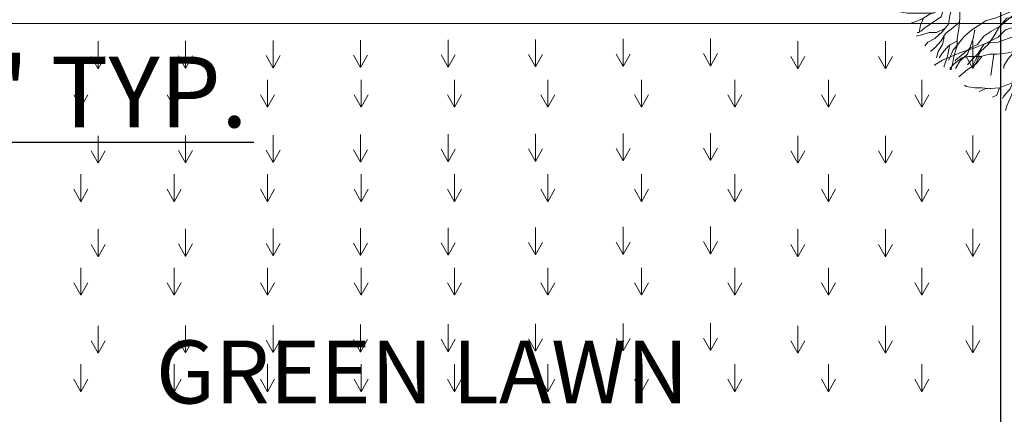
# Model space of a CAD drawing. Units: millimetres. Extents: x 595116 to 630915, y 909473 to 920225.
# Tile 66 of 134: x 629619 to 629744, y 919216 to 919267. Entities that reach past the tile are written whole.
import ezdxf

# ---------------------------------------------------------------- set-up
doc = ezdxf.new("R2010")
doc.units = ezdxf.units.MM
for name, color, linetype, lineweight in [('A-AREA-IDEN', 7, 'Continuous', 20), ('Dimension', 3, 'Continuous', 18), ('L-PLNT', 85, 'Continuous', 13)]:
    doc.layers.add(name, color=color, linetype=linetype, lineweight=lineweight)
doc.styles.get("Standard").update_dxf_attribs({"font": 'arial.ttf'})
doc.dimstyles.new('ISO-25', dxfattribs={"dimtxt": 9, "dimasz": 6, "dimexe": 1.25, "dimexo": 0.625, "dimtad": 1, "dimlunit": 4, "dimtxsty": 'Standard', "dimcen": 2.5, "dimadec": 0, "dimazin": 0, "dimtfac": 1, "dimtmove": 0, "dimatfit": 3, "dimfxl": 1, "dimarcsym": 0})

# ---------------------------------------------------------------- blocks, each defined once
blk = doc.blocks.new('A$C143125F4')
for p, q in [((2.883, 4.834), (2.883, 5.044)), ((2.155, 4.937), (2.117, 4.982)), ((2.21, 4.834), (2.155, 4.937)), ((2.407, 4.879), (2.429, 4.937)), ((2.516, 4.834), (2.538, 4.91)), ((2.538, 4.82), (2.571, 5)), ((2.571, 5), (2.555, 4.982)), ((2.757, 4.892), (2.735, 4.955)), ((1.712, 4.431), (1.712, 4.82)), ((1.822, 4.368), (1.822, 4.802)), ((1.898, 4.776), (1.898, 4.865)), ((1.937, 4.713), (1.991, 4.82)), ((1.991, 4.82), (2.008, 4.865)), ((2.21, 4.744), (2.062, 4.865)), ((2.281, 4.744), (2.21, 4.834)), ((2.298, 4.847), (2.281, 4.892)), ((2.352, 4.758), (2.298, 4.847)), ((2.391, 4.789), (2.407, 4.879)), ((2.391, 4.681), (2.391, 4.789)), ((2.516, 4.52), (2.516, 4.834)), ((2.538, 4.547), (2.538, 4.82)), ((2.648, 4.865), (2.626, 4.892)), ((2.681, 4.776), (2.648, 4.865)), ((2.79, 4.776), (2.757, 4.892)), ((2.867, 4.699), (2.883, 4.834)), ((2.899, 4.699), (2.921, 4.789)), ((2.921, 4.789), (2.96, 4.879)), ((2.96, 4.879), (2.96, 4.892)), ((3.014, 4.713), (3.031, 4.802)), ((3.031, 4.802), (3.031, 4.865)), ((3.047, 4.668), (3.069, 4.789)), ((3.069, 4.789), (3.085, 4.847)), ((3.124, 4.731), (3.124, 4.802)), ((3.178, 4.744), (3.178, 4.82)), ((1.461, 4.681), (1.461, 4.699)), ((1.493, 4.592), (1.461, 4.681)), ((1.625, 4.655), (1.586, 4.699)), ((1.915, 4.668), (1.898, 4.776)), ((1.898, 4.623), (1.937, 4.713)), ((2.298, 4.668), (2.21, 4.744)), ((2.352, 4.578), (2.298, 4.668)), ((2.391, 4.668), (2.352, 4.758)), ((2.429, 4.565), (2.391, 4.668)), ((2.719, 4.681), (2.681, 4.776)), ((2.757, 4.592), (2.719, 4.681)), ((2.812, 4.637), (2.79, 4.776)), ((2.867, 4.431), (2.867, 4.699)), ((2.883, 4.547), (2.899, 4.699)), ((2.976, 4.61), (3.014, 4.713)), ((3.031, 4.578), (3.047, 4.668)), ((3.102, 4.637), (3.124, 4.731)), ((3.156, 4.655), (3.178, 4.744)), ((3.288, 4.637), (3.304, 4.731)), ((3.342, 4.655), (3.375, 4.699)), ((3.414, 4.592), (3.468, 4.681)), ((3.485, 4.623), (3.485, 4.681)), ((1.275, 4.534), (1.258, 4.61)), ((1.368, 4.61), (1.368, 4.623)), ((1.422, 4.52), (1.368, 4.61)), ((1.532, 4.502), (1.493, 4.592)), ((1.658, 4.565), (1.625, 4.655)), ((1.712, 4.475), (1.658, 4.565)), ((1.882, 4.534), (1.898, 4.623)), ((2.429, 4.489), (2.352, 4.578)), ((2.462, 4.444), (2.429, 4.565)), ((2.5, 4.099), (2.538, 4.547)), ((2.79, 4.413), (2.757, 4.592)), ((2.828, 4.296), (2.812, 4.637)), ((2.867, 4.457), (2.883, 4.547)), ((2.976, 4.52), (2.976, 4.61)), ((3.069, 4.457), (3.102, 4.547)), ((3.102, 4.547), (3.102, 4.637)), ((3.14, 4.565), (3.156, 4.655)), ((3.14, 4.413), (3.14, 4.565)), ((3.249, 4.457), (3.266, 4.547)), ((3.266, 4.547), (3.288, 4.637)), ((3.288, 4.565), (3.342, 4.655)), ((3.375, 4.502), (3.414, 4.592)), ((3.507, 4.534), (3.485, 4.623)), ((3.539, 4.444), (3.561, 4.547)), ((3.561, 4.547), (3.578, 4.637)), ((3.578, 4.637), (3.578, 4.655)), ((3.632, 4.534), (3.632, 4.623)), ((1.111, 4.399), (1.039, 4.444)), ((1.056, 4.399), (1.039, 4.431)), ((1.078, 4.457), (1.165, 4.444)), ((1.165, 4.444), (1.258, 4.413)), ((1.368, 4.489), (1.275, 4.534)), ((1.406, 4.341), (1.368, 4.489)), ((1.461, 4.431), (1.422, 4.52)), ((1.548, 4.368), (1.461, 4.431)), ((1.548, 4.413), (1.532, 4.502)), ((1.734, 4.386), (1.712, 4.475)), ((1.822, 4.444), (1.882, 4.534)), ((2.445, 4.399), (2.429, 4.489)), ((2.484, 4.354), (2.462, 4.444)), ((2.5, 4.431), (2.516, 4.52)), ((2.5, 3.458), (2.5, 4.431)), ((2.845, 4.162), (2.867, 4.431)), ((3.047, 4.368), (3.069, 4.457)), ((3.249, 4.368), (3.249, 4.457)), ((3.321, 4.413), (3.375, 4.502)), ((3.507, 4.399), (3.507, 4.534)), ((3.523, 4.31), (3.539, 4.444)), ((3.649, 4.444), (3.632, 4.534)), ((3.649, 4.189), (3.649, 4.444)), ((3.704, 4.413), (3.725, 4.502)), ((3.725, 4.502), (3.725, 4.534)), ((3.797, 4.278), (3.797, 4.489)), ((3.835, 4.386), (3.851, 4.475)), ((3.851, 4.475), (3.868, 4.489)), ((0.946, 4.341), (0.914, 4.386)), ((0.985, 4.251), (0.946, 4.341)), ((1.078, 4.265), (0.985, 4.341)), ((1.094, 4.31), (1.056, 4.399)), ((1.149, 4.22), (1.094, 4.31)), ((1.297, 4.31), (1.111, 4.399)), ((1.258, 4.413), (1.351, 4.386)), ((1.384, 4.278), (1.297, 4.31)), ((1.351, 4.386), (1.439, 4.31)), ((1.439, 4.31), (1.515, 4.22)), ((1.57, 4.296), (1.548, 4.413)), ((1.625, 4.207), (1.57, 4.296)), ((1.767, 4.296), (1.734, 4.386)), ((1.805, 4.207), (1.767, 4.296)), ((1.805, 4.251), (1.822, 4.368)), ((2.5, 4.278), (2.445, 4.399)), ((2.5, 4.265), (2.484, 4.354)), ((2.812, 4.31), (2.79, 4.413)), ((2.828, 4.22), (2.812, 4.31)), ((2.845, 4.207), (2.828, 4.296)), ((3.014, 4.278), (3.047, 4.368)), ((3.069, 4.233), (3.102, 4.323)), ((3.102, 4.323), (3.14, 4.413)), ((3.14, 4.233), (3.211, 4.341)), ((3.211, 4.341), (3.321, 4.413)), ((3.523, 4.31), (3.507, 4.399)), ((3.539, 4.189), (3.523, 4.31)), ((3.671, 4.233), (3.704, 4.413)), ((3.797, 4.278), (3.835, 4.386)), ((3.906, 4.278), (3.961, 4.341)), ((3.961, 4.233), (3.999, 4.323)), ((3.999, 4.323), (3.999, 4.341)), ((0.837, 4.144), (0.766, 4.189)), ((0.837, 4.22), (0.804, 4.265)), ((0.93, 4.175), (0.837, 4.22)), ((1.039, 4.13), (0.93, 4.175)), ((1.039, 4.144), (0.985, 4.251)), ((1.165, 4.175), (1.078, 4.265)), ((1.22, 4.086), (1.165, 4.175)), ((1.493, 4.233), (1.384, 4.278)), ((1.548, 4.144), (1.493, 4.233)), ((1.515, 4.22), (1.603, 4.175)), ((1.603, 4.175), (1.658, 4.086)), ((1.658, 4.099), (1.625, 4.207)), ((1.805, 3.906), (1.805, 4.251)), ((2.516, 4.009), (2.5, 4.278)), ((2.845, 4.117), (2.828, 4.22)), ((2.96, 4.086), (2.992, 4.175)), ((2.992, 4.175), (3.014, 4.278)), ((3.047, 4.189), (3.14, 4.233)), ((3.047, 4.144), (3.069, 4.233)), ((3.561, 4.099), (3.539, 4.189)), ((3.632, 4.144), (3.671, 4.233)), ((3.725, 4.117), (3.813, 4.207)), ((3.78, 4.162), (3.797, 4.278)), ((3.813, 4.207), (3.906, 4.278)), ((3.944, 4.175), (4.037, 4.251)), ((3.944, 4.144), (3.961, 4.233)), ((3.961, 3.92), (4.125, 4.189)), ((4.037, 4.251), (4.037, 4.278)), ((4.125, 4.251), (4.054, 4.162)), ((0.563, 4.027), (0.525, 4.072)), ((0.689, 4.117), (0.673, 4.13)), ((0.782, 4.072), (0.689, 4.117)), ((0.766, 4.086), (0.711, 4.144)), ((0.821, 3.996), (0.766, 4.086)), ((0.968, 4.072), (0.782, 4.072)), ((0.93, 4.099), (0.837, 4.144)), ((1.149, 4.054), (0.968, 4.072)), ((1.132, 4.086), (1.039, 4.13)), ((1.22, 4.054), (1.132, 4.086)), ((1.313, 4.054), (1.22, 4.086)), ((1.313, 4.041), (1.22, 4.054)), ((1.641, 4.054), (1.548, 4.144)), ((1.679, 3.938), (1.641, 4.054)), ((1.658, 4.086), (1.734, 3.996)), ((2.5, 3.996), (2.5, 4.099)), ((2.828, 3.83), (2.845, 4.162)), ((2.938, 3.983), (2.96, 4.086)), ((3.031, 4.054), (3.047, 4.144)), ((3.031, 3.965), (3.031, 4.054)), ((3.594, 4.009), (3.561, 4.099)), ((3.594, 3.875), (3.632, 4.144)), ((3.632, 4.099), (3.725, 4.117)), ((3.922, 4.041), (3.944, 4.144)), ((3.999, 4.072), (3.922, 3.983)), ((4.054, 4.162), (3.999, 4.072)), ((4.147, 3.965), (4.218, 4.054)), ((4.218, 4.054), (4.234, 4.086)), ((0.509, 3.92), (0.509, 3.938)), ((0.602, 3.951), (0.547, 3.996)), ((0.656, 3.983), (0.563, 4.027)), ((0.618, 3.92), (0.563, 3.983)), ((0.635, 3.862), (0.602, 3.951)), ((0.821, 3.965), (0.656, 3.983)), ((0.892, 3.906), (0.821, 3.996)), ((1.406, 4.009), (1.313, 4.041)), ((1.493, 3.996), (1.406, 4.009)), ((1.586, 3.965), (1.493, 3.996)), ((1.679, 3.951), (1.586, 3.965)), ((1.696, 3.817), (1.679, 3.938)), ((1.734, 3.996), (1.789, 3.906)), ((2.883, 3.893), (2.938, 3.983)), ((3.047, 3.875), (3.031, 3.965)), ((3.616, 3.92), (3.594, 4.009)), ((3.922, 3.983), (3.835, 3.92)), ((3.89, 3.951), (3.922, 4.041)), ((4.108, 3.875), (4.147, 3.965)), ((4.147, 3.92), (4.218, 4.009)), ((4.218, 4.009), (4.234, 4.027)), ((4.311, 3.92), (4.344, 3.951)), ((0.47, 3.817), (0.438, 3.83)), ((0.563, 3.741), (0.47, 3.817)), ((0.563, 3.83), (0.509, 3.92)), ((0.602, 3.727), (0.563, 3.83)), ((0.728, 3.862), (0.618, 3.92)), ((0.689, 3.772), (0.635, 3.862)), ((0.914, 3.772), (0.728, 3.862)), ((0.93, 3.817), (0.892, 3.906)), ((0.985, 3.727), (0.93, 3.817)), ((1.734, 3.665), (1.696, 3.817)), ((1.789, 3.906), (1.805, 3.785)), ((2.812, 3.785), (2.883, 3.893)), ((3.14, 3.862), (3.047, 3.875)), ((3.233, 3.83), (3.14, 3.862)), ((3.321, 3.799), (3.233, 3.83)), ((3.578, 3.785), (3.594, 3.875)), ((3.78, 3.83), (3.687, 3.799)), ((3.758, 3.754), (3.961, 3.92)), ((3.835, 3.92), (3.78, 3.83)), ((3.961, 3.785), (4.07, 3.83)), ((4.07, 3.83), (4.147, 3.92)), ((4.125, 3.785), (4.234, 3.83)), ((4.234, 3.83), (4.311, 3.92)), ((4.344, 3.785), (4.437, 3.862)), ((4.437, 3.862), (4.437, 3.893)), ((0.252, 3.696), (0.252, 3.727)), ((0.345, 3.682), (0.252, 3.696)), ((0.492, 3.665), (0.345, 3.682)), ((0.656, 3.696), (0.563, 3.741)), ((0.766, 3.651), (0.656, 3.696)), ((1.023, 3.682), (0.914, 3.772)), ((1.111, 3.62), (1.023, 3.682)), ((1.805, 3.785), (1.805, 3.651)), ((2.757, 3.665), (2.812, 3.785)), ((2.899, 3.638), (2.992, 3.727)), ((2.992, 3.727), (3.102, 3.754)), ((3.102, 3.754), (3.195, 3.772)), ((3.195, 3.772), (3.288, 3.754)), ((3.288, 3.754), (3.375, 3.709)), ((3.414, 3.785), (3.321, 3.799)), ((3.375, 3.709), (3.671, 3.709)), ((3.594, 3.785), (3.414, 3.785)), ((3.687, 3.799), (3.594, 3.785)), ((3.671, 3.709), (3.758, 3.754)), ((3.742, 3.727), (3.835, 3.696)), ((3.835, 3.696), (3.944, 3.665)), ((3.851, 3.696), (3.961, 3.785)), ((3.906, 3.665), (4.015, 3.727)), ((4.015, 3.727), (4.125, 3.785)), ((4.147, 3.785), (4.562, 3.785)), ((4.234, 3.651), (4.344, 3.682)), ((4.344, 3.682), (4.453, 3.696)), ((4.453, 3.696), (4.53, 3.741)), ((0.142, 3.606), (0.126, 3.62)), ((0.235, 3.575), (0.142, 3.606)), ((0.383, 3.561), (0.235, 3.575)), ((0.306, 3.575), (0.306, 3.593)), ((0.399, 3.53), (0.306, 3.575)), ((0.563, 3.561), (0.383, 3.561)), ((0.58, 3.651), (0.492, 3.665)), ((0.766, 3.638), (0.58, 3.651)), ((0.914, 3.638), (0.766, 3.638)), ((1.001, 3.62), (0.914, 3.638)), ((1.204, 3.606), (1.001, 3.62)), ((1.297, 3.561), (1.078, 3.53)), ((1.351, 3.593), (1.204, 3.606)), ((1.422, 3.575), (1.297, 3.561)), ((1.532, 3.53), (1.351, 3.593)), ((1.734, 3.575), (1.734, 3.665)), ((1.767, 3.396), (1.734, 3.575)), ((1.805, 3.651), (1.822, 3.53)), ((2.571, 3.503), (2.664, 3.575)), ((2.626, 3.503), (2.812, 3.593)), ((2.664, 3.575), (2.757, 3.665)), ((2.812, 3.593), (2.899, 3.638)), ((3.944, 3.665), (4.054, 3.651)), ((4.054, 3.651), (4.147, 3.62)), ((4.147, 3.606), (4.234, 3.651)), ((4.147, 3.62), (4.234, 3.593)), ((4.147, 3.62), (4.234, 3.62)), ((4.234, 3.62), (4.344, 3.606)), ((4.234, 3.593), (4.327, 3.548)), ((4.344, 3.606), (4.437, 3.575)), ((4.437, 3.575), (4.546, 3.561)), ((4.453, 3.575), (4.546, 3.62)), ((4.546, 3.62), (4.562, 3.651)), ((4.546, 3.561), (4.601, 3.53)), ((0.345, 3.441), (0.252, 3.427)), ((0.438, 3.458), (0.345, 3.441)), ((0.492, 3.503), (0.399, 3.53)), ((0.525, 3.472), (0.438, 3.458)), ((0.58, 3.472), (0.492, 3.503)), ((0.618, 3.472), (0.525, 3.472)), ((0.711, 3.485), (0.618, 3.472)), ((0.821, 3.503), (0.711, 3.485)), ((0.93, 3.53), (0.821, 3.503)), ((1.078, 3.53), (0.93, 3.53)), ((1.696, 3.517), (1.532, 3.53)), ((1.767, 3.427), (1.696, 3.517)), ((1.822, 3.53), (1.844, 3.414)), ((2.407, 3.351), (2.484, 3.441)), ((2.484, 3.441), (2.571, 3.503)), ((2.555, 3.414), (2.626, 3.503)), ((4.327, 3.548), (4.42, 3.53)), ((4.42, 3.53), (4.53, 3.485)), ((4.53, 3.485), (4.617, 3.441)), ((4.617, 3.441), (4.672, 3.396)), ((0.252, 3.427), (0.219, 3.427)), ((1.789, 3.306), (1.767, 3.396)), ((1.844, 3.414), (1.86, 3.293)), ((2.391, 3.261), (2.407, 3.351)), ((2.484, 3.234), (2.516, 3.324)), ((2.516, 3.324), (2.555, 3.414)), ((1.805, 3.19), (1.789, 3.306)), ((1.822, 3.1), (1.805, 3.19)), ((1.86, 3.293), (1.882, 3.203)), ((1.882, 3.203), (1.882, 3.055)), ((2.374, 3.145), (2.391, 3.261)), ((2.484, 3.145), (2.484, 3.234)), ((4.71, 3.172), (4.727, 3.217)), ((4.71, 3.1), (4.765, 3.19)), ((4.765, 3.19), (4.765, 3.217)), ((1.844, 2.993), (1.822, 3.1)), ((2.374, 3.055), (2.374, 3.145)), ((2.5, 3.055), (2.484, 3.145)), ((4.562, 3.01), (4.655, 3.082)), ((4.655, 3.082), (4.71, 3.172)), ((4.672, 3.01), (4.71, 3.1)), ((4.765, 3.037), (4.781, 3.1)), ((0.164, 2.948), (0.088, 3.024)), ((0.252, 2.89), (0.164, 2.948)), ((1.844, 2.903), (1.844, 2.993)), ((1.882, 3.055), (1.915, 2.961)), ((1.915, 2.961), (1.969, 2.872)), ((2.336, 2.961), (2.374, 3.055)), ((2.336, 2.872), (2.336, 2.961)), ((2.516, 2.961), (2.5, 3.055)), ((2.555, 2.872), (2.516, 2.961)), ((4.508, 2.916), (4.562, 3.01)), ((4.617, 2.845), (4.672, 2.948)), ((4.672, 2.948), (4.765, 3.037)), ((4.727, 2.916), (4.82, 2.979)), ((4.82, 2.979), (4.836, 3.01)), ((0.142, 2.8), (0.071, 2.858)), ((0.109, 2.827), (0.071, 2.858)), ((0.126, 2.903), (0.088, 2.916)), ((0.197, 2.782), (0.109, 2.827)), ((0.219, 2.872), (0.126, 2.903)), ((0.306, 2.845), (0.219, 2.872)), ((0.345, 2.8), (0.252, 2.89)), ((1.86, 2.782), (1.844, 2.903)), ((1.969, 2.872), (2.008, 2.782)), ((2.32, 2.782), (2.336, 2.872)), ((2.626, 2.769), (2.555, 2.872)), ((4.453, 2.813), (4.508, 2.916)), ((4.53, 2.8), (4.639, 2.845)), ((4.639, 2.845), (4.727, 2.845)), ((4.727, 2.845), (4.803, 2.89)), ((4.781, 2.8), (4.836, 2.845)), ((0.142, 2.648), (0.071, 2.737)), ((0.219, 2.71), (0.142, 2.8)), ((0.383, 2.692), (0.197, 2.782)), ((0.29, 2.621), (0.219, 2.71)), ((0.438, 2.737), (0.345, 2.8)), ((0.525, 2.679), (0.438, 2.737)), ((0.711, 2.724), (0.656, 2.782)), ((0.821, 2.666), (0.711, 2.724)), ((1.882, 2.692), (1.86, 2.782)), ((2.008, 2.782), (2.079, 2.692)), ((2.265, 2.692), (2.32, 2.782)), ((2.681, 2.679), (2.626, 2.769)), ((4.382, 2.679), (4.453, 2.813)), ((4.437, 2.769), (4.53, 2.8)), ((4.601, 2.666), (4.694, 2.724)), ((4.694, 2.724), (4.781, 2.8)), ((4.836, 2.692), (4.836, 2.71)), ((0.071, 2.558), (0.016, 2.589)), ((0.033, 2.634), (0.033, 2.648)), ((0.126, 2.589), (0.033, 2.634)), ((0.219, 2.558), (0.126, 2.589)), ((0.219, 2.531), (0.142, 2.648)), ((0.47, 2.692), (0.383, 2.692)), ((0.563, 2.589), (0.525, 2.679)), ((0.635, 2.244), (0.563, 2.589)), ((0.914, 2.603), (0.821, 2.666)), ((1.001, 2.513), (0.914, 2.603)), ((1.991, 2.513), (1.882, 2.692)), ((2.079, 2.692), (2.172, 2.648)), ((2.172, 2.648), (2.265, 2.692)), ((2.774, 2.621), (2.681, 2.679)), ((2.867, 2.603), (2.774, 2.621)), ((2.867, 2.603), (3.085, 2.576)), ((2.96, 2.531), (2.867, 2.603)), ((3.085, 2.576), (3.266, 2.558)), ((3.266, 2.576), (3.375, 2.589)), ((3.375, 2.589), (3.468, 2.621)), ((3.468, 2.621), (3.561, 2.666)), ((3.561, 2.666), (3.578, 2.692)), ((4.272, 2.468), (4.344, 2.576)), ((4.344, 2.576), (4.382, 2.679)), ((4.365, 2.621), (4.453, 2.634)), ((4.453, 2.634), (4.562, 2.648)), ((4.562, 2.648), (4.655, 2.666)), ((4.655, 2.666), (4.748, 2.679)), ((4.748, 2.679), (4.836, 2.692)), ((4.803, 2.558), (4.858, 2.648)), ((0.088, 2.455), (0.033, 2.5)), ((0.164, 2.486), (0.071, 2.558)), ((0.181, 2.424), (0.088, 2.455)), ((0.361, 2.352), (0.219, 2.531)), ((0.892, 2.545), (0.875, 2.558)), ((0.985, 2.5), (0.892, 2.545)), ((1.094, 2.468), (0.985, 2.5)), ((1.242, 2.455), (1.094, 2.468)), ((1.351, 2.424), (1.242, 2.455)), ((1.969, 2.424), (1.991, 2.513)), ((2.845, 2.486), (2.757, 2.442)), ((2.938, 2.442), (2.845, 2.486)), ((3.047, 2.468), (2.96, 2.531)), ((3.14, 2.442), (3.047, 2.468)), ((3.266, 2.558), (3.616, 2.558)), ((3.616, 2.558), (3.797, 2.545)), ((3.797, 2.545), (4.037, 2.545)), ((4.037, 2.545), (4.147, 2.558)), ((4.163, 2.424), (4.272, 2.468)), ((4.617, 2.442), (4.803, 2.558)), ((4.748, 2.442), (4.836, 2.486)), ((4.836, 2.486), (4.874, 2.531)), ((0.071, 2.379), (0, 2.424)), ((0.016, 2.352), (0.126, 2.321)), ((0.164, 2.365), (0.071, 2.379)), ((0.399, 2.334), (0.181, 2.424)), ((0.618, 2.262), (0.399, 2.334)), ((0.837, 2.352), (0.744, 2.307)), ((0.93, 2.41), (0.821, 2.41)), ((0.93, 2.365), (0.837, 2.352)), ((1.023, 2.424), (0.93, 2.41)), ((1.297, 2.365), (0.93, 2.365)), ((1.132, 2.442), (1.023, 2.424)), ((1.351, 2.442), (1.132, 2.442)), ((1.461, 2.352), (1.297, 2.365)), ((1.439, 2.379), (1.351, 2.424)), ((1.548, 2.334), (1.439, 2.379)), ((1.641, 2.244), (1.548, 2.334)), ((1.805, 2.289), (1.882, 2.379)), ((1.882, 2.379), (1.969, 2.424)), ((2.008, 2.397), (1.969, 2.307)), ((2.101, 2.424), (2.008, 2.397)), ((2.21, 2.424), (2.101, 2.424)), ((2.32, 2.442), (2.21, 2.424)), ((2.429, 2.424), (2.32, 2.442)), ((2.516, 2.41), (2.429, 2.424)), ((2.538, 2.321), (2.516, 2.41)), ((2.757, 2.442), (2.719, 2.352)), ((2.719, 2.352), (2.735, 2.262)), ((2.992, 2.352), (2.938, 2.442)), ((3.069, 2.262), (2.992, 2.352)), ((3.233, 2.365), (3.14, 2.442)), ((3.288, 2.276), (3.233, 2.365)), ((4.015, 2.262), (4.054, 2.365)), ((4.054, 2.365), (4.163, 2.424)), ((4.344, 2.307), (4.53, 2.397)), ((4.53, 2.397), (4.617, 2.442)), ((4.584, 2.424), (4.913, 2.424)), ((4.601, 2.321), (4.694, 2.379)), ((4.694, 2.379), (4.781, 2.379)), ((4.781, 2.379), (4.858, 2.41)), ((0.055, 2.262), (0, 2.307)), ((0.088, 2.186), (0.033, 2.218)), ((0.164, 2.244), (0.055, 2.262)), ((0.126, 2.321), (0.235, 2.321)), ((0.252, 2.218), (0.164, 2.244)), ((0.235, 2.321), (0.328, 2.307)), ((0.361, 2.2), (0.252, 2.218)), ((0.328, 2.307), (0.416, 2.276)), ((0.416, 2.276), (0.602, 2.276)), ((0.602, 2.276), (0.689, 2.244)), ((0.689, 2.244), (0.782, 2.231)), ((0.782, 2.231), (0.875, 2.186)), ((1.625, 2.2), (1.712, 2.231)), ((1.712, 2.231), (1.805, 2.289)), ((1.882, 2.244), (1.767, 2.2)), ((1.969, 2.307), (1.882, 2.244)), ((2.538, 1.873), (2.538, 2.321)), ((2.735, 2.262), (2.812, 2.173)), ((3.178, 2.186), (3.069, 2.262)), ((3.375, 2.218), (3.288, 2.276)), ((3.452, 2.123), (3.375, 2.218)), ((3.414, 2.186), (3.507, 2.231)), ((3.507, 2.231), (3.616, 2.231)), ((3.616, 2.231), (3.835, 2.244)), ((3.835, 2.244), (3.999, 2.262)), ((3.999, 2.262), (4.147, 2.262)), ((4.147, 2.262), (4.256, 2.276)), ((4.256, 2.276), (4.344, 2.307)), ((4.327, 2.307), (4.891, 2.307)), ((4.891, 2.307), (4.984, 2.289)), ((4.984, 2.289), (4.984, 2.276)), ((0.181, 2.141), (0.088, 2.186)), ((0.274, 2.052), (0.181, 2.141)), ((0.673, 2.2), (0.361, 2.2)), ((0.525, 2.097), (0.416, 2.02)), ((0.618, 2.186), (0.525, 2.097)), ((0.766, 2.173), (0.673, 2.2)), ((0.859, 2.123), (0.766, 2.173)), ((0.875, 1.989), (0.859, 2.123)), ((0.875, 2.186), (0.914, 2.097)), ((0.914, 2.097), (0.946, 2.007)), ((1.439, 2.079), (1.532, 2.141)), ((1.532, 2.141), (1.625, 2.2)), ((1.696, 2.11), (1.586, 2.052)), ((1.767, 2.2), (1.696, 2.11)), ((2.664, 2.123), (2.626, 2.034)), ((2.757, 2.079), (2.664, 2.123)), ((2.812, 2.173), (2.845, 2.079)), ((3.249, 2.097), (3.178, 2.186)), ((3.342, 2.034), (3.249, 2.097)), ((3.539, 2.065), (3.452, 2.123)), ((4.344, 2.079), (4.475, 2.123)), ((4.475, 2.123), (4.655, 2.155)), ((4.508, 2.123), (4.617, 2.123)), ((4.617, 2.123), (4.803, 2.097)), ((4.655, 2.155), (4.858, 2.186)), ((4.803, 2.097), (4.82, 2.065)), ((4.858, 2.186), (4.874, 2.186)), ((0.109, 2.052), (0.055, 2.034)), ((0.219, 1.976), (0.088, 1.976)), ((0.454, 2.052), (0.109, 2.052)), ((0.328, 1.962), (0.219, 1.976)), ((0.416, 2.02), (0.328, 1.944)), ((0.875, 1.841), (0.875, 1.989)), ((0.946, 2.007), (0.985, 1.917)), ((1.258, 1.944), (1.351, 2.007)), ((1.351, 2.007), (1.439, 2.079)), ((1.493, 2.007), (1.384, 1.917)), ((1.586, 2.052), (1.493, 2.007)), ((2.538, 1.989), (2.5, 1.899)), ((2.626, 2.034), (2.609, 1.944)), ((2.774, 1.989), (2.757, 2.079)), ((2.828, 1.899), (2.774, 1.989)), ((2.845, 2.079), (2.867, 1.989)), ((2.867, 1.989), (2.921, 1.899)), ((3.397, 1.944), (3.342, 2.034)), ((3.632, 2.007), (3.539, 2.065)), ((3.725, 1.976), (3.632, 2.007)), ((3.835, 1.962), (3.725, 1.976)), ((3.922, 1.976), (3.835, 1.962)), ((4.015, 1.944), (3.922, 1.976)), ((4.108, 1.976), (4.015, 1.944)), ((4.201, 1.989), (4.108, 1.976)), ((4.125, 1.989), (4.234, 2.052)), ((4.201, 1.976), (4.201, 1.989)), ((4.672, 1.976), (4.201, 1.976)), ((4.234, 2.052), (4.344, 2.079)), ((4.584, 1.944), (4.694, 1.962)), ((4.765, 1.989), (4.672, 1.976)), ((4.694, 1.962), (4.803, 1.976)), ((4.82, 1.962), (4.727, 1.931)), ((4.858, 2.052), (4.765, 1.989)), ((4.803, 1.976), (4.858, 1.989)), ((0.219, 1.886), (0.126, 1.828)), ((0.274, 1.886), (0.181, 1.796)), ((0.328, 1.944), (0.219, 1.886)), ((0.821, 1.752), (0.875, 1.841)), ((0.985, 1.917), (0.985, 1.828)), ((1.078, 1.828), (1.165, 1.886)), ((1.165, 1.886), (1.258, 1.944)), ((1.384, 1.917), (1.297, 1.81)), ((2.5, 1.899), (2.298, 1.752)), ((2.516, 1.783), (2.538, 1.873)), ((2.609, 1.855), (2.593, 1.765)), ((2.609, 1.944), (2.609, 1.855)), ((2.899, 1.81), (2.828, 1.899)), ((2.921, 1.899), (2.992, 1.81)), ((3.485, 1.917), (3.397, 1.944)), ((3.414, 1.917), (3.507, 1.886)), ((3.578, 1.886), (3.485, 1.917)), ((3.507, 1.886), (3.578, 1.796)), ((3.671, 1.873), (3.578, 1.886)), ((3.758, 1.855), (3.671, 1.873)), ((3.851, 1.841), (3.758, 1.855)), ((3.944, 1.841), (3.851, 1.841)), ((4.037, 1.855), (3.944, 1.841)), ((4.125, 1.855), (4.037, 1.855)), ((4.53, 1.855), (4.125, 1.855)), ((4.218, 1.855), (4.311, 1.873)), ((4.311, 1.873), (4.398, 1.917)), ((4.327, 1.841), (4.453, 1.796)), ((4.398, 1.917), (4.491, 1.917)), ((4.491, 1.917), (4.584, 1.944)), ((4.617, 1.886), (4.53, 1.855)), ((4.727, 1.931), (4.617, 1.886)), ((0.126, 1.828), (0.088, 1.796)), ((0.181, 1.796), (0.142, 1.738)), ((0.219, 1.72), (0.142, 1.675)), ((0.328, 1.752), (0.219, 1.72)), ((0.454, 1.72), (0.306, 1.649)), ((0.438, 1.765), (0.328, 1.752)), ((0.837, 1.765), (0.438, 1.765)), ((0.618, 1.765), (0.454, 1.72)), ((0.728, 1.662), (0.821, 1.752)), ((1.149, 1.752), (0.968, 1.693)), ((0.985, 1.828), (1.078, 1.828)), ((1.149, 1.752), (1.078, 1.662)), ((1.297, 1.81), (1.149, 1.752)), ((2.298, 1.752), (2.188, 1.662)), ((2.538, 1.796), (2.462, 1.693)), ((2.516, 1.693), (2.516, 1.783)), ((2.593, 1.765), (2.593, 1.393)), ((2.976, 1.72), (2.899, 1.81)), ((3.069, 1.649), (2.976, 1.72)), ((2.992, 1.81), (3.085, 1.738)), ((3.085, 1.738), (3.195, 1.559)), ((3.578, 1.796), (3.687, 1.752)), ((3.687, 1.752), (3.78, 1.72)), ((3.78, 1.72), (3.999, 1.662)), ((4.453, 1.796), (4.546, 1.752)), ((4.546, 1.752), (4.639, 1.675)), ((4.617, 1.81), (4.71, 1.796)), ((4.71, 1.796), (4.781, 1.765)), ((0.197, 1.604), (0.126, 1.572)), ((0.306, 1.649), (0.197, 1.604)), ((0.399, 1.675), (0.328, 1.586)), ((0.525, 1.559), (0.635, 1.604)), ((0.782, 1.617), (0.602, 1.559)), ((0.635, 1.604), (0.728, 1.662)), ((0.968, 1.693), (0.782, 1.617)), ((1.078, 1.662), (1.001, 1.572)), ((1.023, 1.617), (1.023, 1.514)), ((2.101, 1.617), (2.024, 1.528)), ((2.188, 1.662), (2.101, 1.617)), ((2.462, 1.693), (2.391, 1.572)), ((2.5, 1.559), (2.516, 1.693)), ((3.102, 1.541), (3.069, 1.649)), ((3.868, 1.693), (3.944, 1.572)), ((3.999, 1.662), (4.179, 1.586)), ((4.07, 1.631), (4.163, 1.617)), ((4.163, 1.617), (4.53, 1.617)), ((4.53, 1.617), (4.617, 1.604)), ((4.617, 1.604), (4.71, 1.617)), ((4.639, 1.675), (4.71, 1.631)), ((0.274, 1.425), (0.345, 1.514)), ((0.306, 1.496), (0.274, 1.438)), ((0.328, 1.586), (0.306, 1.496)), ((0.345, 1.514), (0.438, 1.541)), ((0.509, 1.483), (0.399, 1.407)), ((0.438, 1.541), (0.525, 1.559)), ((0.602, 1.559), (0.509, 1.483)), ((1.001, 1.572), (0.914, 1.451)), ((1.023, 1.514), (1.001, 1.393)), ((2.024, 1.528), (1.937, 1.451)), ((2.391, 1.572), (2.336, 1.438)), ((2.462, 1.469), (2.5, 1.559)), ((3.124, 1.451), (3.102, 1.541)), ((3.195, 1.559), (3.211, 1.469)), ((3.944, 1.572), (4.037, 1.469)), ((3.999, 1.528), (4.108, 1.451)), ((4.179, 1.586), (4.272, 1.559)), ((4.218, 1.572), (4.311, 1.528)), ((4.272, 1.559), (4.42, 1.541)), ((4.311, 1.528), (4.398, 1.483)), ((4.398, 1.483), (4.475, 1.38)), ((4.42, 1.541), (4.508, 1.496)), ((4.475, 1.514), (4.672, 1.514)), ((4.508, 1.496), (4.584, 1.407)), ((0.29, 1.38), (0.252, 1.362)), ((0.399, 1.407), (0.29, 1.38)), ((0.728, 1.362), (0.618, 1.317)), ((0.914, 1.451), (0.728, 1.362)), ((0.804, 1.407), (0.766, 1.286)), ((0.914, 1.438), (0.875, 1.304)), ((1.001, 1.393), (1.001, 1.272)), ((1.658, 1.362), (1.439, 1.272)), ((1.751, 1.38), (1.658, 1.362)), ((1.844, 1.407), (1.696, 1.335)), ((1.844, 1.425), (1.751, 1.38)), ((1.915, 1.38), (1.805, 1.286)), ((1.937, 1.451), (1.844, 1.425)), ((1.937, 1.469), (1.915, 1.38)), ((2.243, 1.38), (2.101, 1.317)), ((2.336, 1.438), (2.243, 1.286)), ((2.391, 1.286), (2.445, 1.38)), ((2.445, 1.38), (2.462, 1.469)), ((2.593, 1.393), (2.484, 1.214)), ((3.156, 1.362), (3.124, 1.451)), ((3.233, 1.183), (3.156, 1.362)), ((3.211, 1.469), (3.233, 1.38)), ((3.233, 1.38), (3.249, 1.241)), ((4.037, 1.469), (4.125, 1.393)), ((4.108, 1.451), (4.218, 1.407)), ((4.108, 1.393), (4.201, 1.362)), ((4.125, 1.393), (4.179, 1.286)), ((4.201, 1.362), (4.289, 1.335)), ((4.218, 1.407), (4.311, 1.393)), ((4.311, 1.393), (4.398, 1.362)), ((4.398, 1.362), (4.491, 1.317)), ((4.475, 1.38), (4.546, 1.286)), ((0.345, 1.335), (0.252, 1.348)), ((0.673, 1.335), (0.345, 1.335)), ((0.438, 1.227), (0.399, 1.214)), ((0.525, 1.259), (0.438, 1.227)), ((0.547, 1.272), (0.509, 1.183)), ((0.618, 1.317), (0.525, 1.259)), ((0.673, 1.227), (0.563, 1.151)), ((0.766, 1.286), (0.673, 1.227)), ((0.875, 1.304), (0.859, 1.196)), ((1.001, 1.227), (0.914, 1.151)), ((1.001, 1.272), (0.985, 1.138)), ((1.329, 1.241), (1.242, 1.183)), ((1.439, 1.272), (1.329, 1.241)), ((1.696, 1.335), (1.493, 1.169)), ((1.586, 1.272), (1.493, 1.169)), ((1.751, 1.286), (1.586, 1.272)), ((1.805, 1.286), (1.696, 1.169)), ((1.898, 1.304), (1.751, 1.286)), ((2.101, 1.317), (1.898, 1.304)), ((2.062, 1.241), (1.953, 1.151)), ((2.134, 1.335), (2.062, 1.241)), ((2.243, 1.286), (2.172, 1.183)), ((2.391, 1.227), (2.227, 0.959)), ((2.391, 1.196), (2.391, 1.286)), ((3.249, 1.241), (3.266, 1.151)), ((4.179, 1.286), (4.272, 1.227)), ((4.201, 1.241), (4.218, 1.124)), ((4.272, 1.227), (4.344, 1.138)), ((4.289, 1.335), (4.382, 1.272)), ((4.382, 1.272), (4.475, 1.227)), ((4.475, 1.227), (4.508, 1.214)), ((4.491, 1.317), (4.546, 1.286)), ((0.509, 1.183), (0.492, 1.093)), ((0.563, 1.151), (0.509, 1.107)), ((0.782, 1.107), (0.689, 1.017)), ((0.804, 1.138), (0.711, 1.093)), ((0.859, 1.196), (0.782, 1.107)), ((0.914, 1.151), (0.821, 1.08)), ((0.985, 1.138), (0.968, 1.017)), ((1.149, 1.124), (1.056, 1.048)), ((1.242, 1.183), (1.149, 1.124)), ((1.187, 1.124), (1.165, 1.017)), ((1.384, 1.107), (1.297, 1.048)), ((1.493, 1.169), (1.384, 1.107)), ((1.493, 1.169), (1.422, 1.048)), ((1.57, 1.124), (1.477, 1.035)), ((1.696, 1.169), (1.57, 1.124)), ((1.953, 1.151), (1.86, 1.062)), ((2.172, 1.183), (2.062, 1.048)), ((2.374, 1.107), (2.391, 1.196)), ((2.374, 1.017), (2.374, 1.107)), ((2.445, 1.124), (2.407, 1.093)), ((2.484, 1.214), (2.445, 1.124)), ((3.266, 1.003), (3.233, 1.183)), ((3.266, 1.151), (3.304, 1.062)), ((3.304, 1.107), (3.342, 1.017)), ((4.218, 1.124), (4.234, 1.035)), ((4.344, 1.138), (4.398, 1.048)), ((0.525, 1.062), (0.454, 1.048)), ((0.492, 1.093), (0.47, 1.093)), ((0.618, 1.093), (0.525, 1.062)), ((0.689, 1.017), (0.602, 0.972)), ((0.711, 1.093), (0.618, 1.093)), ((0.766, 0.99), (0.689, 0.9)), ((0.821, 1.08), (0.766, 0.99)), ((0.804, 1.035), (0.782, 0.945)), ((0.968, 0.99), (0.859, 0.927)), ((1.056, 1.048), (0.914, 0.869)), ((0.968, 1.017), (0.968, 0.927)), ((1.165, 1.017), (1.132, 0.927)), ((1.297, 1.048), (1.22, 0.945)), ((1.384, 0.99), (1.297, 0.945)), ((1.422, 1.048), (1.351, 0.945)), ((1.477, 1.035), (1.384, 0.99)), ((1.679, 1.048), (1.477, 0.972)), ((1.86, 1.062), (1.679, 1.048)), ((2.062, 1.048), (2.008, 0.927)), ((2.352, 0.927), (2.374, 1.017)), ((2.407, 1.093), (2.391, 1.003)), ((2.391, 1.003), (2.391, 0.676)), ((2.429, 1.08), (2.445, 0.959)), ((3.249, 1.08), (3.249, 0.587)), ((3.304, 0.914), (3.266, 1.003)), ((3.304, 1.062), (3.321, 0.959)), ((3.342, 1.017), (3.43, 0.972)), ((4.218, 1.08), (4.311, 1.08)), ((4.234, 1.035), (4.272, 0.945)), ((4.311, 1.08), (4.382, 1.035)), ((4.398, 1.048), (4.42, 1.035)), ((0.602, 0.972), (0.563, 0.927)), ((0.689, 0.9), (0.635, 0.856)), ((0.782, 0.945), (0.728, 0.856)), ((0.859, 0.927), (0.782, 0.838)), ((0.875, 0.945), (0.859, 0.856)), ((0.914, 0.869), (0.875, 0.779)), ((0.968, 0.927), (0.93, 0.811)), ((1.132, 0.9), (0.946, 0.748)), ((1.187, 0.9), (1.001, 0.838)), ((1.132, 0.927), (1.094, 0.824)), ((1.22, 0.945), (1.132, 0.9)), ((1.329, 0.959), (1.187, 0.9)), ((1.297, 0.945), (1.22, 0.824)), ((1.351, 0.945), (1.258, 0.856)), ((1.477, 0.972), (1.329, 0.959)), ((1.789, 0.883), (1.603, 0.838)), ((1.991, 0.927), (1.789, 0.883)), ((2.008, 0.927), (1.953, 0.824)), ((2.227, 0.959), (2.155, 0.838)), ((2.352, 0.838), (2.352, 0.927)), ((2.445, 0.959), (2.462, 0.869)), ((2.462, 0.869), (2.5, 0.735)), ((3.321, 0.824), (3.304, 0.914)), ((3.321, 0.959), (3.375, 0.869)), ((3.375, 0.869), (3.43, 0.748)), ((3.43, 0.972), (3.523, 0.959)), ((3.523, 0.959), (3.632, 0.945)), ((3.632, 0.945), (3.742, 0.945)), ((3.687, 0.945), (3.742, 0.856)), ((3.742, 0.945), (3.851, 0.927)), ((3.851, 0.927), (3.961, 0.9)), ((3.961, 0.9), (4.054, 0.869)), ((4.054, 0.869), (4.147, 0.856)), ((4.272, 0.945), (4.289, 0.9)), ((0.782, 0.748), (0.689, 0.69)), ((0.728, 0.856), (0.711, 0.779)), ((0.782, 0.838), (0.744, 0.779)), ((1.001, 0.838), (0.782, 0.748)), ((0.837, 0.766), (0.804, 0.676)), ((0.859, 0.856), (0.837, 0.766)), ((0.875, 0.779), (0.859, 0.748)), ((0.93, 0.811), (0.914, 0.721)), ((1.023, 0.779), (0.93, 0.703)), ((0.946, 0.748), (0.946, 0.735)), ((1.094, 0.824), (1.001, 0.735)), ((1.111, 0.793), (1.023, 0.779)), ((1.258, 0.793), (1.111, 0.793)), ((1.22, 0.824), (1.132, 0.735)), ((1.204, 0.766), (1.165, 0.69)), ((1.258, 0.856), (1.204, 0.766)), ((1.275, 0.793), (1.204, 0.703)), ((1.368, 0.824), (1.258, 0.793)), ((1.461, 0.824), (1.368, 0.824)), ((1.422, 0.824), (1.384, 0.556)), ((1.603, 0.838), (1.461, 0.824)), ((1.603, 0.766), (1.548, 0.676)), ((1.679, 0.856), (1.603, 0.766)), ((1.953, 0.824), (1.86, 0.703)), ((2.117, 0.748), (2.024, 0.614)), ((2.155, 0.838), (2.117, 0.748)), ((2.352, 0.824), (2.298, 0.735)), ((2.336, 0.748), (2.352, 0.838)), ((2.336, 0.39), (2.336, 0.748)), ((3.359, 0.735), (3.321, 0.824)), ((3.43, 0.748), (3.539, 0.659)), ((3.742, 0.856), (3.851, 0.811)), ((3.851, 0.811), (3.944, 0.766)), ((3.906, 0.793), (3.999, 0.779)), ((3.944, 0.766), (4.015, 0.676)), ((3.999, 0.779), (4.092, 0.793)), ((4.092, 0.793), (4.179, 0.779)), ((4.147, 0.856), (4.201, 0.824)), ((0.689, 0.69), (0.689, 0.676)), ((0.804, 0.676), (0.804, 0.659)), ((0.93, 0.703), (0.875, 0.645)), ((0.892, 0.632), (0.875, 0.632)), ((0.914, 0.721), (0.892, 0.632)), ((1.001, 0.735), (0.946, 0.645)), ((1.094, 0.632), (0.985, 0.542)), ((1.132, 0.735), (1.094, 0.69)), ((1.204, 0.703), (1.094, 0.632)), ((1.548, 0.676), (1.548, 0.645)), ((1.767, 0.614), (1.679, 0.524)), ((1.822, 0.659), (1.751, 0.542)), ((1.86, 0.703), (1.767, 0.614)), ((2.024, 0.632), (1.937, 0.542)), ((2.024, 0.614), (1.953, 0.524)), ((2.281, 0.645), (2.265, 0.511)), ((2.298, 0.735), (2.281, 0.645)), ((2.391, 0.676), (2.374, 0.569)), ((2.5, 0.735), (2.538, 0.645)), ((2.516, 0.659), (2.609, 0.542)), ((2.538, 0.645), (2.648, 0.466)), ((3.452, 0.645), (3.359, 0.735)), ((3.397, 0.703), (3.414, 0.614)), ((3.414, 0.614), (3.578, 0.345)), ((3.539, 0.569), (3.452, 0.645)), ((3.539, 0.676), (3.78, 0.645)), ((3.539, 0.659), (3.649, 0.587)), ((3.78, 0.645), (3.944, 0.632)), ((3.944, 0.632), (4.037, 0.645)), ((4.015, 0.676), (4.054, 0.659)), ((1.679, 0.524), (1.625, 0.39)), ((1.751, 0.542), (1.696, 0.403)), ((1.953, 0.524), (1.789, 0.255)), ((1.937, 0.542), (1.822, 0.452)), ((2.265, 0.511), (2.227, 0.376)), ((2.374, 0.569), (2.374, 0.452)), ((2.407, 0.511), (2.407, 0.421)), ((2.609, 0.542), (2.757, 0.466)), ((3.249, 0.587), (3.304, 0.497)), ((3.249, 0.587), (3.266, 0.497)), ((3.266, 0.497), (3.288, 0.403)), ((3.304, 0.497), (3.375, 0.403)), ((3.485, 0.497), (3.485, 0.376)), ((3.725, 0.452), (3.539, 0.569)), ((3.578, 0.556), (3.649, 0.466)), ((3.649, 0.587), (3.742, 0.524)), ((3.742, 0.524), (3.835, 0.479)), ((1.078, 0.421), (1.056, 0.435)), ((1.187, 0.403), (1.078, 0.421)), ((1.275, 0.403), (1.187, 0.403)), ((1.313, 0.39), (1.242, 0.358)), ((1.384, 0.39), (1.275, 0.403)), ((1.493, 0.403), (1.313, 0.39)), ((1.493, 0.403), (1.461, 0.314)), ((1.679, 0.479), (1.493, 0.403)), ((1.625, 0.39), (1.548, 0.3)), ((1.696, 0.403), (1.641, 0.314)), ((1.822, 0.452), (1.767, 0.358)), ((1.898, 0.39), (1.86, 0.255)), ((1.953, 0.479), (1.898, 0.39)), ((1.915, 0.376), (1.915, 0.287)), ((2.227, 0.376), (2.21, 0.242)), ((2.32, 0.3), (2.336, 0.39)), ((2.352, 0.358), (2.374, 0.479)), ((2.374, 0.479), (2.352, 0.376)), ((2.374, 0.452), (2.352, 0.358)), ((2.352, 0.376), (2.352, 0.345)), ((2.407, 0.421), (2.445, 0.332)), ((2.648, 0.466), (2.719, 0.376)), ((2.719, 0.376), (2.757, 0.287)), ((2.757, 0.466), (2.899, 0.421)), ((2.845, 0.421), (2.867, 0.332)), ((2.899, 0.421), (3.014, 0.376)), ((3.014, 0.376), (3.102, 0.358)), ((3.288, 0.403), (3.321, 0.224)), ((3.342, 0.452), (3.375, 0.358)), ((3.375, 0.403), (3.452, 0.314)), ((3.485, 0.376), (3.507, 0.287)), ((3.649, 0.466), (3.725, 0.376)), ((3.813, 0.421), (3.725, 0.452)), ((3.725, 0.376), (3.725, 0.358)), ((3.835, 0.479), (3.868, 0.466)), ((1.461, 0.314), (1.406, 0.287)), ((1.548, 0.3), (1.532, 0.269)), ((1.641, 0.314), (1.586, 0.179)), ((1.696, 0.269), (1.658, 0.224)), ((1.767, 0.358), (1.696, 0.269)), ((1.789, 0.255), (1.712, 0.197)), ((1.86, 0.255), (1.86, 0.166)), ((1.915, 0.287), (1.937, 0.197)), ((2.227, 0.332), (2.172, 0.242)), ((2.21, 0.255), (2.188, 0.134)), ((2.32, 0.211), (2.32, 0.3)), ((2.352, 0.345), (2.336, 0.255)), ((2.336, 0.255), (2.336, 0)), ((2.445, 0.332), (2.462, 0.242)), ((2.484, 0.269), (2.571, 0.211)), ((2.719, 0.314), (2.735, 0.211)), ((2.757, 0.287), (2.812, 0.197)), ((2.867, 0.332), (2.96, 0.269)), ((2.96, 0.269), (3.047, 0.179)), ((3.102, 0.358), (3.195, 0.287)), ((3.195, 0.287), (3.266, 0.224)), ((3.375, 0.358), (3.414, 0.269)), ((3.414, 0.269), (3.43, 0.242)), ((3.578, 0.345), (3.594, 0.314)), ((1.586, 0.179), (1.57, 0.121)), ((1.86, 0.166), (1.822, 0.121)), ((1.937, 0.197), (1.937, 0.09)), ((2.101, 0.152), (2.024, 0.121)), ((2.172, 0.242), (2.101, 0.152)), ((2.134, 0.152), (2.101, 0.076)), ((2.21, 0.242), (2.134, 0.152)), ((2.188, 0.134), (2.172, 0.09)), ((2.298, 0.121), (2.32, 0.211)), ((2.462, 0.242), (2.5, 0.152)), ((2.5, 0.166), (2.484, 0.076)), ((2.5, 0.152), (2.516, 0.063)), ((2.571, 0.211), (2.648, 0.121)), ((2.735, 0.211), (2.774, 0.121)), ((2.79, 0.242), (2.899, 0.197)), ((2.812, 0.197), (2.899, 0.108)), ((2.899, 0.197), (2.976, 0.108)), ((3.047, 0.179), (3.085, 0.166)), ((3.321, 0.224), (3.342, 0.197)), ((2.298, 0.018), (2.298, 0.121)), ((2.484, 0.076), (2.462, 0.045)), ((2.516, 0.063), (2.516, 0.045)), ((2.648, 0.121), (2.702, 0.045)), ((2.774, 0.121), (2.812, 0.063)), ((2.899, 0.108), (2.976, 0.031)), ((2.976, 0.108), (3.014, 0.076))]:
    blk.add_line(p, q)
blk = doc.blocks.new('LAWN-GRASS-TUFT')
blk.add_line((0.89, 3.49), (0.89, 0))
blk.add_lwpolyline([(0, 1.58), (0.89, 0), (1.78, 1.58)])
blk = doc.blocks.new('*D211')
at = {"layer": 'Defpoints', "color": 0, "transparency": 16777216}
for p in [(629535.39, 919258.66), (629586.23, 919258.66), (629586.23, 919250.94)]:
    blk.add_point(p, dxfattribs=at)
at = {"layer": 'Dimension', "color": 0, "lineweight": -2, "transparency": 16777216}
for p, q in [((629535.39, 919258.04), (629535.39, 919249.69)), ((629586.23, 919258.04), (629586.23, 919249.69)), ((629541.39, 919250.94), (629580.23, 919250.94)), ((629586.23, 919250.94), (629648.7, 919250.94))]:
    blk.add_line(p, q, dxfattribs=at)
at = {"layer": 'Dimension', "color": 0, "transparency": 16777216}
for points in [[(629541.39, 919251.94), (629541.39, 919249.94), (629535.39, 919250.94)], [(629580.23, 919251.94), (629580.23, 919249.94), (629586.23, 919250.94)]]:
    blk.add_solid(points, dxfattribs=at)
at = {"layer": 'Dimension', "color": 0, "transparency": 16777216, "insert": (629620.46, 919256.17), "char_height": 9, "attachment_point": 5}
blk.add_mtext('4\'-3" TYP.', dxfattribs=at)
blk = doc.blocks.new('*D216')
at = {"layer": 'Defpoints', "color": 0, "transparency": 16777216}
for p in [(629505.04, 919411.83), (629743.54, 919411.93), (629743.54, 918832.38)]:
    blk.add_point(p, dxfattribs=at)
at = {"layer": 'Dimension', "color": 0, "lineweight": -2, "transparency": 16777216}
for p, q in [((629505.04, 919411.2), (629505.04, 918831.13)), ((629743.54, 919411.3), (629743.54, 918831.13)), ((629511.04, 918832.38), (629737.54, 918832.38))]:
    blk.add_line(p, q, dxfattribs=at)
at = {"layer": 'Dimension', "color": 0, "transparency": 16777216}
for points in [[(629511.04, 918833.38), (629511.04, 918831.38), (629505.04, 918832.38)], [(629737.54, 918833.38), (629737.54, 918831.38), (629743.54, 918832.38)]]:
    blk.add_solid(points, dxfattribs=at)
at = {"layer": 'Dimension', "color": 0, "transparency": 16777216, "insert": (629624.29, 918837.66), "char_height": 9, "attachment_point": 5}
blk.add_mtext('19\'-10 1/2"', dxfattribs=at)

msp = doc.modelspace()

# ---------------------------------------------------------------- linework, layer by layer
at = {"layer": 'L-PLNT'}
msp.add_line((629800.951, 919266.009), (629535.274, 919266.009), dxfattribs=at)

# ---------------------------------------------------------------- block references
at = {"layer": 'L-PLNT', "xscale": 10.20167662382051, "yscale": 10.20167662382051, "zscale": 10.20167662382051}
msp.add_blockref('A$C143125F4', (629728.194, 919253.739), dxfattribs=at)
at = {"layer": 'L-PLNT'}
for p in [(629628.026, 919260.275), (629639.139, 919260.324), (629650.253, 919260.374), (629661.367, 919260.423), (629672.481, 919260.473), (629683.595, 919260.522), (629694.708, 919260.572), (629705.822, 919260.622), (629716.936, 919260.275), (629728.05, 919260.275), (629739.164, 919260.324), (629625.811, 919255.397), (629637.684, 919255.397), (629649.557, 919255.397), (629661.43, 919255.397), (629673.303, 919255.397), (629685.176, 919255.397), (629697.049, 919255.397), (629708.922, 919255.397), (629720.795, 919255.397), (629732.669, 919255.397), (629628.026, 919248.272), (629639.139, 919248.322), (629650.253, 919248.371), (629661.367, 919248.421), (629672.481, 919248.47), (629683.595, 919248.52), (629694.708, 919248.57), (629705.822, 919248.619), (629716.936, 919248.272), (629728.05, 919248.272), (629739.164, 919248.322), (629625.811, 919243.395), (629637.684, 919243.395), (629649.557, 919243.395), (629661.43, 919243.395), (629673.303, 919243.395), (629685.176, 919243.395), (629697.049, 919243.395), (629708.922, 919243.395), (629720.795, 919243.395), (629732.669, 919243.395), (629650.253, 919236.497), (629661.367, 919236.546), (629672.481, 919236.596), (629683.595, 919236.645), (629694.708, 919236.695), (629705.822, 919236.745), (629628.026, 919236.398), (629639.139, 919236.447), (629716.936, 919236.398), (629728.05, 919236.398), (629739.164, 919236.447), (629625.811, 919231.52), (629637.684, 919231.52), (629649.557, 919231.52), (629661.43, 919231.52), (629673.303, 919231.52), (629685.176, 919231.52), (629697.049, 919231.52), (629708.922, 919231.52), (629720.795, 919231.52), (629732.669, 919231.52), (629628.026, 919224.142), (629639.139, 919224.191), (629650.253, 919224.241), (629661.367, 919224.291), (629672.481, 919224.34), (629683.595, 919224.39), (629694.708, 919224.439), (629705.822, 919224.489), (629716.936, 919224.142), (629728.05, 919224.142), (629739.164, 919224.191), (629625.811, 919219.264), (629637.684, 919219.264), (629649.557, 919219.264), (629661.43, 919219.264), (629673.303, 919219.264), (629685.176, 919219.264), (629697.049, 919219.264), (629708.922, 919219.264), (629720.795, 919219.264), (629732.669, 919219.264)]:
    msp.add_blockref('LAWN-GRASS-TUFT', p, dxfattribs=at)

# ---------------------------------------------------------------- texts
at = {"layer": 'A-AREA-IDEN', "insert": (629628.918, 919225.763), "char_height": 8, "attachment_point": 1}
msp.add_mtext_dynamic_manual_height_columns('{   GREEN LAWN}', width=83.57324, gutter_width=12.5, heights=[0], dxfattribs=at)

# ---------------------------------------------------------------- dimensions: what is measured, and where the dimension line sits
at = {"layer": 'Dimension'}
dim = msp.add_linear_dim(base=(629743.541, 918832.378), p1=(629505.041, 919411.828), p2=(629743.541, 919411.928), dimstyle='ISO-25', override={"dimdec": 1, "dimlfac": 1, "dimrnd": 0, "dimzin": 1, "dimdsep": 46, "dimlunit": 4, "dimfrac": 2}, dxfattribs=at)
dim.commit()
dim.dimension.update_dxf_attribs({"geometry": '*D216', "text_midpoint": (629624.291, 918837.656)})
dim = msp.add_linear_dim(base=(629586.227, 919250.943), p1=(629535.386, 919258.662), p2=(629586.227, 919258.662), text='<> TYP.', dimstyle='ISO-25', override={"dimdec": 1, "dimlfac": 1, "dimrnd": 0, "dimzin": 1, "dimdsep": 46, "dimlunit": 4, "dimfrac": 2}, dxfattribs=at)
dim.commit()
dim.dimension.update_dxf_attribs({"geometry": '*D211', "text_midpoint": (629620.463, 919256.167)})

doc.saveas('drawing.dxf')
